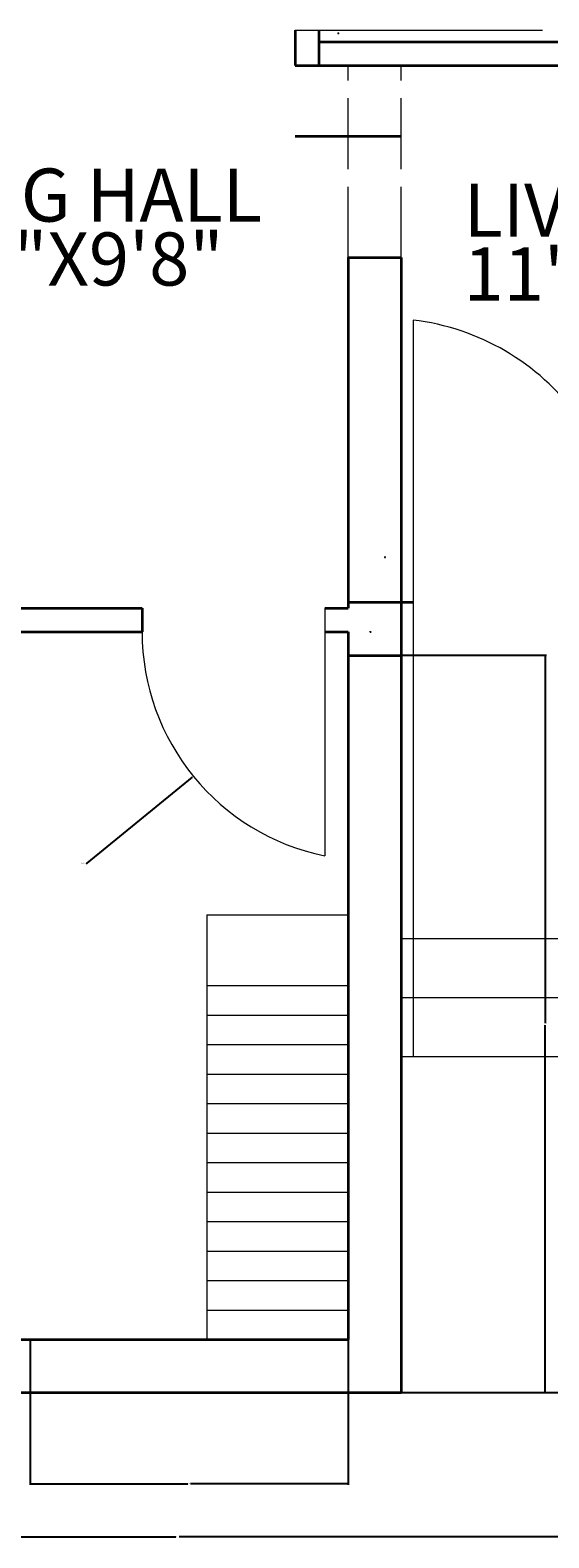
# Model space of a CAD drawing. Units: inches. Extents: x 2473 to 3664, y 1231 to 2079.
# Tile 4 of 8: x 2782 to 2870, y 1563 to 1819. Entities that reach past the tile are written whole.
import ezdxf

# ---------------------------------------------------------------- set-up
doc = ezdxf.new("R2010")
doc.units = ezdxf.units.IN
doc.linetypes.add('ACAD_ISO02W100', pattern=[15, 12, -3])
doc.layers.get('Defpoints').update_dxf_attribs({"linetype": 'ACAD_ISO02W100'})
for name, color, linetype, lineweight in [('A-ANNO-DIMS', 2, 'Continuous', 18), ('A-AREA-IDEN', 7, 'Continuous', 18), ('A-DOOR', 4, 'Continuous', 18), ('A-FLOR-CASE', 9, 'Continuous', 18), ('A-FLOR-STRS', 7, 'Continuous', 18), ('A-WALL', 7, 'Continuous', 35), ('A-WALL-OVHD', 7, 'ACAD_ISO02W100', 18)]:
    doc.layers.add(name, color=color, linetype=linetype, lineweight=lineweight)
doc.styles.get("Standard").update_dxf_attribs({"font": 'arial.ttf'})
doc.dimstyles.get("Standard").update_dxf_attribs({"dimtxt": 0.18, "dimasz": 0.18, "dimexe": 0.18, "dimexo": 0.0625, "dimgap": 0.09, "dimtad": 0, "dimtih": 1, "dimtoh": 1, "dimdec": 4, "dimzin": 0, "dimdsep": 46, "dimtxsty": 'Standard', "dimcen": 0.09, "dimadec": 0, "dimazin": 0, "dimtfac": 1, "dimtdec": 4, "dimtofl": 0, "dimtmove": 0, "dimatfit": 3, "dimfxl": 1, "dimtolj": 1, "dimtzin": 0, "dimarcsym": 0})

# ---------------------------------------------------------------- blocks, each defined once
blk = doc.blocks.new('STEPS-SITOUT-PLAN')
for p, q in [((151, 68), (151, 0)), ((0, 20), (151, 20)), ((0, 10), (151, 10)), ((0, 0), (151, 0))]:
    blk.add_line(p, q)
blk = doc.blocks.new('*D49')
at = {"layer": 'A-ANNO-DIMS', "color": 0, "lineweight": -2, "transparency": 16777216}
for p, q in [((2995.66, 1644.99), (2995.66, 1563.43)), ((2617.66, 1587.99), (2617.66, 1563.43)), ((2617.84, 1563.61), (2806.37, 1563.61)), ((2995.48, 1563.61), (2806.95, 1563.61))]:
    blk.add_line(p, q, dxfattribs=at)
at = {"layer": 'A-ANNO-DIMS', "color": 0, "transparency": 16777216}
for points in [[(2617.84, 1563.64), (2617.84, 1563.58), (2617.66, 1563.61)], [(2995.48, 1563.64), (2995.48, 1563.58), (2995.66, 1563.61)]]:
    blk.add_solid(points, dxfattribs=at)
at = {"layer": 'Defpoints', "color": 0, "transparency": 16777216}
for p in [(2995.66, 1645.06), (2617.66, 1588.06), (2995.66, 1563.61)]:
    blk.add_point(p, dxfattribs=at)
at = {"layer": 'A-ANNO-DIMS', "color": 0, "transparency": 16777216, "insert": (2806.66, 1563.61), "char_height": 0.18, "attachment_point": 5}
blk.add_mtext('\\A1;378', dxfattribs=at)
blk = doc.blocks.new('*D50')
at = {"layer": 'A-ANNO-DIMS', "color": 0, "lineweight": -2, "transparency": 16777216}
for p, q in [((2746.72, 2006.06), (3020.29, 2006.06)), ((3020.11, 2005.88), (3020.11, 1797.24)), ((3020.11, 1588.24), (3020.11, 1796.87)), ((2844.72, 1588.06), (3020.29, 1588.06))]:
    blk.add_line(p, q, dxfattribs=at)
at = {"layer": 'A-ANNO-DIMS', "color": 0, "transparency": 16777216}
for points in [[(3020.08, 2005.88), (3020.14, 2005.88), (3020.11, 2006.06)], [(3020.08, 1588.24), (3020.14, 1588.24), (3020.11, 1588.06)]]:
    blk.add_solid(points, dxfattribs=at)
at = {"layer": 'Defpoints', "color": 0, "transparency": 16777216}
for p in [(2746.66, 2006.06), (3020.11, 2006.06), (2844.66, 1588.06)]:
    blk.add_point(p, dxfattribs=at)
at = {"layer": 'A-ANNO-DIMS', "color": 0, "transparency": 16777216, "insert": (3020.11, 1797.06), "char_height": 0.18, "attachment_point": 5}
blk.add_mtext('\\A1;418', dxfattribs=at)
blk = doc.blocks.new('*D52')
at = {"layer": 'A-ANNO-DIMS', "color": 0, "lineweight": -2, "transparency": 16777216}
for p, q in [((2844.72, 1713.06), (2869.29, 1713.06)), ((2869.11, 1712.88), (2869.11, 1650.74)), ((2869.11, 1588.24), (2869.11, 1650.37)), ((2844.72, 1588.06), (2869.29, 1588.06))]:
    blk.add_line(p, q, dxfattribs=at)
at = {"layer": 'A-ANNO-DIMS', "color": 0, "transparency": 16777216}
for points in [[(2869.08, 1712.88), (2869.14, 1712.88), (2869.11, 1713.06)], [(2869.08, 1588.24), (2869.14, 1588.24), (2869.11, 1588.06)]]:
    blk.add_solid(points, dxfattribs=at)
at = {"layer": 'Defpoints', "color": 0, "transparency": 16777216}
for p in [(2844.66, 1713.06), (2844.66, 1588.06), (2869.11, 1588.06)]:
    blk.add_point(p, dxfattribs=at)
at = {"layer": 'A-ANNO-DIMS', "color": 0, "transparency": 16777216, "insert": (2869.11, 1650.56), "char_height": 0.18, "attachment_point": 5}
blk.add_mtext('\\A1;125', dxfattribs=at)
blk = doc.blocks.new('*D56')
at = {"layer": 'A-ANNO-DIMS', "color": 0, "lineweight": -2, "transparency": 16777216}
for p, q in [((2781.66, 1596.99), (2781.66, 1572.43)), ((2835.66, 1596.99), (2835.66, 1572.43)), ((2781.84, 1572.61), (2808.44, 1572.61)), ((2835.48, 1572.61), (2808.88, 1572.61))]:
    blk.add_line(p, q, dxfattribs=at)
at = {"layer": 'A-ANNO-DIMS', "color": 0, "transparency": 16777216}
for points in [[(2781.84, 1572.64), (2781.84, 1572.58), (2781.66, 1572.61)], [(2835.48, 1572.64), (2835.48, 1572.58), (2835.66, 1572.61)]]:
    blk.add_solid(points, dxfattribs=at)
at = {"layer": 'Defpoints', "color": 0, "transparency": 16777216}
for p in [(2781.66, 1597.06), (2835.66, 1597.06), (2781.66, 1572.61)]:
    blk.add_point(p, dxfattribs=at)
at = {"layer": 'A-ANNO-DIMS', "color": 0, "transparency": 16777216, "insert": (2808.66, 1572.61), "char_height": 0.18, "attachment_point": 5}
blk.add_mtext('\\A1;54', dxfattribs=at)
blk = doc.blocks.new('*D105')
at = {"layer": 'A-ANNO-DIMS', "color": 0, "lineweight": -2, "transparency": 16777216}
for p, q in [((2894.18, 1767.94), (2874.73, 1753.71)), ((2894.36, 1767.94), (2894.18, 1767.94)), ((2841.83, 1729.71), (2842.01, 1729.71)), ((2841.92, 1729.62), (2841.92, 1729.8))]:
    blk.add_line(p, q, dxfattribs=at)
at = {"layer": 'A-ANNO-DIMS', "color": 0, "transparency": 16777216}
blk.add_solid([(2874.71, 1753.73), (2874.75, 1753.68), (2874.58, 1753.6)], dxfattribs=at)
at = {"layer": 'Defpoints', "color": 0, "transparency": 16777216}
for p in [(2874.58, 1753.6), (2841.92, 1729.71)]:
    blk.add_point(p, dxfattribs=at)
at = {"layer": 'A-ANNO-DIMS', "color": 0, "transparency": 16777216, "insert": (2894.84, 1767.94), "char_height": 0.18, "attachment_point": 5}
blk.add_mtext('\\A1;R40.47', dxfattribs=at)
blk = doc.blocks.new('*D106')
at = {"layer": 'A-ANNO-DIMS', "color": 0, "lineweight": -2, "transparency": 16777216}
for p, q in [((2839.36, 1717.06), (2839.54, 1717.06)), ((2839.45, 1716.97), (2839.45, 1717.15)), ((2791.36, 1677.82), (2809.25, 1692.42)), ((2791.18, 1677.82), (2791.36, 1677.82))]:
    blk.add_line(p, q, dxfattribs=at)
at = {"layer": 'A-ANNO-DIMS', "color": 0, "transparency": 16777216}
blk.add_solid([(2809.23, 1692.45), (2809.27, 1692.4), (2809.39, 1692.54)], dxfattribs=at)
at = {"layer": 'Defpoints', "color": 0, "transparency": 16777216}
for p in [(2839.45, 1717.06), (2809.39, 1692.54)]:
    blk.add_point(p, dxfattribs=at)
at = {"layer": 'A-ANNO-DIMS', "color": 0, "transparency": 16777216, "insert": (2790.7, 1677.82), "char_height": 0.18, "attachment_point": 5}
blk.add_mtext('\\A1;R38.79', dxfattribs=at)
blk = doc.blocks.new('*D108')
at = {"layer": 'A-ANNO-DIMS', "color": 0, "lineweight": -2, "transparency": 16777216}
for p, q in [((2870.98, 1859.89), (2857.23, 1844.52)), ((2871.16, 1859.89), (2870.98, 1859.89)), ((2833.9, 1818.54), (2834.08, 1818.54)), ((2833.99, 1818.45), (2833.99, 1818.63))]:
    blk.add_line(p, q, dxfattribs=at)
at = {"layer": 'A-ANNO-DIMS', "color": 0, "transparency": 16777216}
blk.add_solid([(2857.21, 1844.54), (2857.25, 1844.5), (2857.11, 1844.38)], dxfattribs=at)
at = {"layer": 'Defpoints', "color": 0, "transparency": 16777216}
for p in [(2857.11, 1844.38), (2833.99, 1818.54)]:
    blk.add_point(p, dxfattribs=at)
at = {"layer": 'A-ANNO-DIMS', "color": 0, "transparency": 16777216, "insert": (2871.64, 1859.89), "char_height": 0.18, "attachment_point": 5}
blk.add_mtext('\\A1;R34.68', dxfattribs=at)

msp = doc.modelspace()

# ---------------------------------------------------------------- linework, layer by layer
at = {"layer": 'A-DOOR'}
for p, q in [((2826.6604, 1819.0561), (2868.6604, 1819.0561)), ((2846.6604, 1769.8992), (2846.6604, 1722.0561)), ((2831.6604, 1721.0561), (2831.6604, 1679.0561))]:
    msp.add_line(p, q, dxfattribs=at)
for centre, radius, start, end in [((2841.9202, 1729.7076), 40.4701, 349.101732, 83.273573), ((2839.4507, 1717.0561), 38.7903, 180, 258.414407)]:
    msp.add_arc(centre, radius, start, end, dxfattribs=at)
at = {"layer": 'A-FLOR-CASE'}
for p, q in [((2811.6604, 1669.0561), (2811.6604, 1597.0561)), ((2811.6604, 1669.0561), (2835.6604, 1669.0561)), ((2811.6604, 1657.0561), (2835.6604, 1657.0561)), ((2811.6604, 1652.0561), (2835.6604, 1652.0561)), ((2811.6604, 1647.0561), (2835.6604, 1647.0561)), ((2811.6604, 1642.0561), (2835.6604, 1642.0561)), ((2811.6604, 1637.0561), (2835.6604, 1637.0561)), ((2811.6604, 1632.0561), (2835.6604, 1632.0561)), ((2811.6604, 1627.0561), (2835.6604, 1627.0561)), ((2811.6604, 1622.0561), (2835.6604, 1622.0561)), ((2811.6604, 1617.0561), (2835.6604, 1617.0561)), ((2811.6604, 1617.0561), (2835.6604, 1617.0561)), ((2811.6604, 1612.0561), (2835.6604, 1612.0561)), ((2811.6604, 1607.0561), (2835.6604, 1607.0561)), ((2811.6604, 1602.0561), (2835.6604, 1602.0561))]:
    msp.add_line(p, q, dxfattribs=at)
at = {"layer": 'A-FLOR-STRS'}
msp.add_line((2846.6604, 1722.0561), (2846.6604, 1645.0561), dxfattribs=at)
at = {"layer": 'A-WALL'}
for p, q in [((2826.6604, 1819.0561), (2826.6604, 1813.0561)), ((2826.6604, 1819.0561), (2826.6604, 1813.0561)), ((2830.6604, 1819.0561), (2830.6604, 1813.0561)), ((2830.6604, 1819.0561), (2830.6604, 1813.0561)), ((2830.6604, 1819.0561), (2830.6604, 1813.0561)), ((2830.6604, 1817.0561), (2995.6604, 1817.0561)), ((2826.6604, 1813.0561), (2986.6604, 1813.0561)), ((2826.6604, 1801.0561), (2844.6604, 1801.0561)), ((2835.6604, 1780.5146), (2844.6604, 1780.5146)), ((2835.6604, 1780.5146), (2835.6604, 1721.0561)), ((2844.6604, 1780.5146), (2844.6604, 1588.0561)), ((2844.6604, 1761.0561), (2844.6604, 1713.0561)), ((2688.6604, 1721.0561), (2800.6604, 1721.0561)), ((2800.6604, 1721.0561), (2800.6604, 1717.0561)), ((2831.6604, 1721.0561), (2835.6604, 1721.0561)), ((2835.6604, 1722.0561), (2846.6604, 1722.0561)), ((2844.6604, 1722.0561), (2844.6604, 1588.0561)), ((2692.6604, 1717.0561), (2800.6604, 1717.0561)), ((2831.6604, 1717.0561), (2835.6604, 1717.0561)), ((2835.6604, 1717.0561), (2835.6604, 1597.0561)), ((2835.6604, 1713.0561), (2844.6604, 1713.0561)), ((2835.6604, 1713.0561), (2835.6604, 1597.0561)), ((2692.6604, 1597.0561), (2835.6604, 1597.0561)), ((2617.6604, 1588.0561), (2844.6604, 1588.0561))]:
    msp.add_line(p, q, dxfattribs=at)
at = {"layer": 'A-WALL-OVHD'}
for p, q in [((2835.6604, 1780.5146), (2835.6604, 1813.0561)), ((2844.6604, 1780.5146), (2844.6604, 1813.0561))]:
    msp.add_line(p, q, dxfattribs=at)

# ---------------------------------------------------------------- block references
at = {"layer": 'A-FLOR-STRS'}
msp.add_blockref('STEPS-SITOUT-PLAN', (2844.66, 1645.056), dxfattribs=at)

# ---------------------------------------------------------------- texts
at = {"layer": 'A-AREA-IDEN'}
for s, p in [('DINING HALL', (2746.6787, 1786.5949)), (' LIVING', (2852.4886, 1784.047)), ('   16\'8"X9\'8"', (2746.6787, 1775.7567)), (' 11\'X8\'4"', (2852.4886, 1773.2089))]:
    msp.add_text(s, height=9, dxfattribs=at).set_placement(p)

# ---------------------------------------------------------------- dimensions: what is measured, and where the dimension line sits
at = {"layer": 'A-ANNO-DIMS'}
for base, p1, p2, angle, picture, middle in [((3020.1104, 2006.0561), (2844.6604, 1588.0561), (2746.6604, 2006.0561), 90, '*D50', (3020.1104, 1797.0561)), ((2869.1104, 1588.0561), (2844.6604, 1713.0561), (2844.6604, 1588.0561), 270, '*D52', (2869.1104, 1650.5561)), ((2781.6604, 1572.6061), (2835.6604, 1597.0561), (2781.6604, 1597.0561), 180, '*D56', (2808.6604, 1572.6061))]:
    dim = msp.add_linear_dim(base=base, p1=p1, p2=p2, angle=angle, dimstyle='Standard', override={"dimdec": 0, "dimlfac": 1, "dimrnd": 0, "dimzin": 0, "dimdsep": 46, "dimlunit": 2}, dxfattribs=at)
    dim.commit()
    dim.dimension.update_dxf_attribs({"geometry": picture, "text_midpoint": middle})
for center, mpoint, picture, middle in [((2833.9877, 1818.5395), (2857.1099, 1844.3819), '*D108', (2871.6433, 1859.8873)), ((2841.9202, 1729.7076), (2874.5833, 1753.6022), '*D105', (2894.841, 1767.939)), ((2839.4507, 1717.0561), (2809.3931, 1692.5361), '*D106', (2790.6986, 1677.8241))]:
    dim = msp.add_radius_dim(center=center, mpoint=mpoint, dimstyle='Standard', override={"dimdec": 2, "dimlfac": 1, "dimrnd": 0, "dimzin": 0, "dimdsep": 46, "dimlunit": 2}, dxfattribs=at)
    dim.commit()
    dim.dimension.update_dxf_attribs({"geometry": picture, "text_midpoint": middle, "dimtype": 164})
dim = msp.add_linear_dim(base=(2995.6604, 1563.6061), p1=(2617.6604, 1588.0561), p2=(2995.6604, 1645.0561), dimstyle='Standard', override={"dimdec": 0, "dimlfac": 1, "dimrnd": 0, "dimzin": 0, "dimdsep": 46, "dimlunit": 2}, dxfattribs=at)
dim.commit()
dim.dimension.update_dxf_attribs({"geometry": '*D49', "text_midpoint": (2806.6604, 1563.6061)})

doc.saveas('drawing.dxf')
